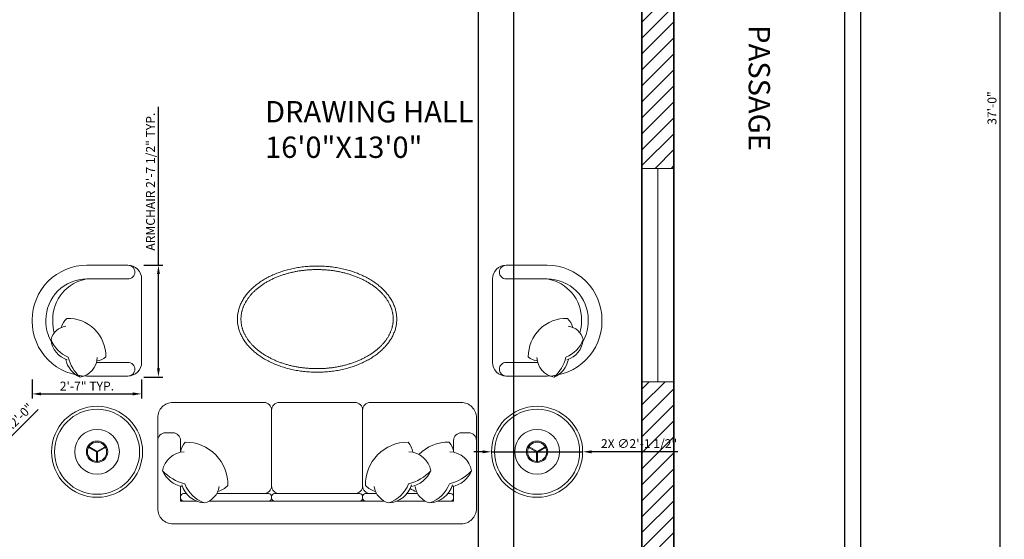
# Model space of a CAD drawing. Units: inches. Extents: x 3618 to 4156, y 1271 to 2023.
# Tile 3 of 5: x 3879 to 4156, y 1488 to 1635. Entities that reach past the tile are written whole.
import ezdxf

# ---------------------------------------------------------------- set-up
doc = ezdxf.new("R2010")
doc.units = ezdxf.units.IN
for name, color, linetype, lineweight in [('A-ANNO-DIMS', 2, 'Continuous', 18), ('A-AREA-IDEN', 7, 'Continuous', 18), ('A-FURN', 8, 'Continuous', 18), ('A-GLAZ', 4, 'Continuous', 18), ('A-WALL', 7, 'Continuous', 35), ('A-WALL-PATT', 252, 'Continuous', 13), ('C-PROP', 7, 'Continuous', 25)]:
    doc.layers.add(name, color=color, linetype=linetype, lineweight=lineweight)
doc.styles.get("Standard").update_dxf_attribs({"font": 'arial.ttf'})
doc.dimstyles.new('ISO-25', dxfattribs={"dimtxt": 2.5, "dimasz": 2.5, "dimexe": 1.25, "dimexo": 0.625, "dimtad": 1, "dimdec": 0, "dimlunit": 3, "dimtxsty": 'Standard', "dimcen": 2.5, "dimadec": 0, "dimazin": 0, "dimtfac": 1, "dimtdec": 0, "dimtmove": 0, "dimatfit": 3, "dimfxl": 1, "dimarcsym": 0})

# ---------------------------------------------------------------- blocks, each defined once
blk = doc.blocks.new('WINDOW-60X9')
for p, q in [((0, 60), (0, 0)), ((9, 60), (0, 60)), ((4.5, 60), (4.5, 0)), ((9, 0), (9, 60)), ((0, 0), (9, 0))]:
    blk.add_line(p, q)
blk = doc.blocks.new('ARMCHAIR')
at = {"ltscale": 0.03}
blk.add_lwpolyline([(30.78, 15.9), (30.78, 27.63, 0.414214), (26.93, 31.48), (15.39, 31.48, 0.414214), (0, 16.09), (0, 15.9), (0, 15.71, 0.414214), (15.39, 0.31), (26.93, 0.31, 0.414214), (30.78, 4.16), (30.78, 15.9)], format="xyb", dxfattribs=at)
for points in [[(15.39, 27.63), (26.93, 27.63, 0.414214), (28.86, 29.56), (28.86, 29.56, 0.414214), (26.93, 31.48)], [(15.39, 27.63, 0.414214), (3.85, 16.09), (3.85, 15.9)], [(15.39, 27.63, 0.372719), (5.77, 16.09), (5.77, 15.9)], [(5.37, 9.98, -0.130591), (3.85, 15.71), (3.85, 15.9)], [(9.88, 4.85, -0.306663), (5.29, 10.58, -0.30633), (9.48, 14.33, 0.872847)], [(6.19, 12.43, -0.072384), (5.77, 15.71), (5.77, 15.9)], [(18.18, 4.54, 0.165541), (20.72, 5.73, 0.425989), (9.7, 16.54, 0.121523), (8.18, 13.97, -7.115464)], [(13.45, 0, -0.14773), (10.14, 5.62, -0.213343), (5.29, 10.58, -0.178662)], [(18.3, 5.51, -0.356772), (13.45, 0, -0.249542), (9.45, 4.99, 9.61688)], [(18.09, 4.16), (26.93, 4.16, -0.414214), (28.86, 2.24), (28.86, 2.24, -0.414214), (26.93, 0.31)]]:
    blk.add_lwpolyline(points, format="xyb")
blk = doc.blocks.new('TABLE-END-ROUND')
at = {"ltscale": 0.03}
for p, q in [((-0.07, -0.12), (-2.67, 1.39)), ((0.07, 0.12), (-2.54, 1.62)), ((-0.13, 0), (-0.13, -3.01)), ((-0.07, 0.12), (2.54, 1.62)), ((0.07, -0.12), (2.67, 1.39)), ((0.13, 0), (0.13, -3.01))]:
    blk.add_line(p, q, dxfattribs=at)
for radius in [12.8, 6.29, 3.01, 2.7]:
    blk.add_circle((0, 0), radius, dxfattribs=at)
blk.add_circle((0, 0), 11.95)
blk = doc.blocks.new('*D40')
at = {"layer": 'A-ANNO-DIMS', "color": 0, "lineweight": -2, "transparency": 16777216}
for p, q in [((3918.22, 1565.57), (3918.22, 1610.13)), ((3914.12, 1565.57), (3919.47, 1565.57)), ((3918.22, 1536.59), (3918.22, 1563.07)), ((3914.12, 1534.09), (3919.47, 1534.09))]:
    blk.add_line(p, q, dxfattribs=at)
at = {"layer": 'A-ANNO-DIMS', "color": 0, "transparency": 16777216}
for points in [[(3917.81, 1563.07), (3918.64, 1563.07), (3918.22, 1565.57)], [(3917.81, 1536.59), (3918.64, 1536.59), (3918.22, 1534.09)]]:
    blk.add_solid(points, dxfattribs=at)
at = {"layer": 'Defpoints', "color": 0, "transparency": 16777216}
for p in [(3913.5, 1565.57), (3918.22, 1565.57), (3913.5, 1534.09)]:
    blk.add_point(p, dxfattribs=at)
at = {"layer": 'A-ANNO-DIMS', "color": 0, "transparency": 16777216, "insert": (3916.3, 1589.1), "char_height": 2.5, "attachment_point": 5, "rotation": 90}
blk.add_mtext('ARMCHAIR 2\'-7 1/2" TYP.', dxfattribs=at)
blk = doc.blocks.new('*D41')
at = {"layer": 'A-ANNO-DIMS', "color": 0, "lineweight": -2, "transparency": 16777216}
for p, q in [((3882.72, 1533.47), (3882.72, 1528.12)), ((3913.5, 1533.47), (3913.5, 1528.12)), ((3885.22, 1529.37), (3911, 1529.37))]:
    blk.add_line(p, q, dxfattribs=at)
at = {"layer": 'A-ANNO-DIMS', "color": 0, "transparency": 16777216}
for points in [[(3885.22, 1529.79), (3885.22, 1528.95), (3882.72, 1529.37)], [(3911, 1529.79), (3911, 1528.95), (3913.5, 1529.37)]]:
    blk.add_solid(points, dxfattribs=at)
at = {"layer": 'Defpoints', "color": 0, "transparency": 16777216}
for p in [(3882.72, 1534.09), (3913.5, 1534.09), (3913.5, 1529.37)]:
    blk.add_point(p, dxfattribs=at)
at = {"layer": 'A-ANNO-DIMS', "color": 0, "transparency": 16777216, "insert": (3898.11, 1531.25), "char_height": 2.5, "attachment_point": 5}
blk.add_mtext('2\'-7" TYP.', dxfattribs=at)
blk = doc.blocks.new('*D53')
at = {"layer": 'A-ANNO-DIMS', "color": 0, "lineweight": -2, "transparency": 16777216}
for p, q in [((4008.19, 1440.44), (4008.19, 1974.21)), ((4018.19, 1440.44), (4018.19, 1974.21)), ((4010.69, 1972.96), (4015.69, 1972.96))]:
    blk.add_line(p, q, dxfattribs=at)
at = {"layer": 'A-ANNO-DIMS', "color": 0, "transparency": 16777216}
for points in [[(4010.69, 1973.38), (4010.69, 1972.54), (4008.19, 1972.96)], [(4015.69, 1973.38), (4015.69, 1972.54), (4018.19, 1972.96)]]:
    blk.add_solid(points, dxfattribs=at)
at = {"layer": 'Defpoints', "color": 0, "transparency": 16777216}
for p in [(4018.19, 1972.96), (4008.19, 1439.81), (4018.19, 1439.81)]:
    blk.add_point(p, dxfattribs=at)
at = {"layer": 'A-ANNO-DIMS', "color": 0, "transparency": 16777216, "insert": (4013.19, 1974.86), "char_height": 2.5, "attachment_point": 5}
blk.add_mtext('0\'-10"', dxfattribs=at)
blk = doc.blocks.new('*D56')
at = {"layer": 'A-ANNO-DIMS', "color": 0, "lineweight": -2, "transparency": 16777216}
for p, q in [((4063.81, 1831.81), (4156.09, 1831.81)), ((4154.84, 1829.31), (4154.84, 1390.31)), ((4063.81, 1387.81), (4156.09, 1387.81))]:
    blk.add_line(p, q, dxfattribs=at)
at = {"layer": 'A-ANNO-DIMS', "color": 0, "transparency": 16777216}
for points in [[(4154.42, 1829.31), (4155.25, 1829.31), (4154.84, 1831.81)], [(4154.42, 1390.31), (4155.25, 1390.31), (4154.84, 1387.81)]]:
    blk.add_solid(points, dxfattribs=at)
at = {"layer": 'Defpoints', "color": 0, "transparency": 16777216}
for p in [(4063.19, 1831.81), (4063.19, 1387.81), (4154.84, 1387.81)]:
    blk.add_point(p, dxfattribs=at)
at = {"layer": 'A-ANNO-DIMS', "color": 0, "transparency": 16777216, "insert": (4152.94, 1609.81), "char_height": 2.5, "attachment_point": 5, "rotation": 90}
blk.add_mtext('37\'-0"', dxfattribs=at)
blk = doc.blocks.new('*D60')
at = {"layer": 'A-ANNO-DIMS', "color": 0, "lineweight": -2, "transparency": 16777216}
for p, q in [((4009.41, 1513.08), (4006.91, 1513.08)), ((4011.91, 1513.08), (4037.51, 1513.08)), ((4064.24, 1513.08), (4040.01, 1513.08))]:
    blk.add_line(p, q, dxfattribs=at)
at = {"layer": 'A-ANNO-DIMS', "color": 0, "transparency": 16777216}
for points in [[(4009.41, 1513.49), (4009.41, 1512.66), (4011.91, 1513.08)], [(4040.01, 1513.49), (4040.01, 1512.66), (4037.51, 1513.08)]]:
    blk.add_solid(points, dxfattribs=at)
at = {"layer": 'Defpoints', "color": 0, "transparency": 16777216}
for p in [(4011.91, 1513.08), (4037.51, 1513.08)]:
    blk.add_point(p, dxfattribs=at)
at = {"layer": 'A-ANNO-DIMS', "color": 0, "transparency": 16777216, "insert": (4053.38, 1515.05), "char_height": 2.5, "attachment_point": 5, "rotation": 359.9984}
blk.add_mtext('2X ∅2\'-1 1/2"', dxfattribs=at)
blk = doc.blocks.new('*D62')
at = {"layer": 'A-ANNO-DIMS', "color": 0, "lineweight": -2, "transparency": 16777216}
for p, q in [((3884.38, 1525), (3870.43, 1511.05)), ((3851.69, 1492.31), (3868.66, 1509.28))]:
    blk.add_line(p, q, dxfattribs=at)
at = {"layer": 'A-ANNO-DIMS', "color": 0, "transparency": 16777216}
blk.add_solid([(3870.13, 1511.34), (3870.72, 1510.75), (3868.66, 1509.28)], dxfattribs=at)
at = {"layer": 'Defpoints', "color": 0, "transparency": 16777216}
for p in [(3868.66, 1509.28), (3851.69, 1492.31)]:
    blk.add_point(p, dxfattribs=at)
at = {"layer": 'A-ANNO-DIMS', "color": 0, "transparency": 16777216, "insert": (3877.5, 1520.81), "char_height": 2.5, "attachment_point": 5, "rotation": 45.0011}
blk.add_mtext('3X R2\'-0"', dxfattribs=at)

msp = doc.modelspace()

# ---------------------------------------------------------------- hatches: boundary and pattern name
at = {"layer": 'A-WALL-PATT'}
h = msp.add_hatch(dxfattribs=at)
h.set_pattern_fill('ANSI31', color=256)
h.paths.add_polyline_path([(4115.69, 1933.81), (3704.69, 1933.81), (3704.69, 1885.81), (3713.69, 1885.81), (3713.69, 1924.81), (4115.69, 1924.81)])
h.paths.add_polyline_path([(3886.19, 1924.81), (3881.69, 1924.81), (3881.69, 1786.81), (3875.69, 1786.81), (3875.69, 1782.31), (3892.19, 1782.31), (3892.19, 1786.81), (3886.19, 1786.81)])
h.paths.add_polyline_path([(3763.69, 1784.56), (3763.69, 1786.81), (3713.69, 1786.81), (3713.69, 1782.31), (3763.69, 1782.31)], flags=17)
h.paths.add_polyline_path([(3713.69, 1825.81), (3704.69, 1825.81), (3704.69, 1764.31), (3713.69, 1764.31)])
h.paths.add_polyline_path([(3802.19, 1782.31), (3835.69, 1782.31), (3835.69, 1784.56), (3835.69, 1786.81), (3791.69, 1786.81), (3791.69, 1782.31), (3797.69, 1782.31), (3797.69, 1722.31), (3713.69, 1722.31), (3713.69, 1717.81), (3797.69, 1717.81), (3797.69, 1657.81), (3791.69, 1657.81), (3791.69, 1653.31), (3851.69, 1653.31), (3851.69, 1647.31), (3856.19, 1647.31), (3856.19, 1657.81), (3802.19, 1657.81)])
h.paths.add_polyline_path([(3713.69, 1740.31), (3704.69, 1740.31), (3704.69, 1699.81), (3713.69, 1699.81)])
h.paths.add_polyline_path([(3713.69, 1675.81), (3704.69, 1675.81), (3704.69, 1623.31), (3713.69, 1623.31)])
h.paths.add_polyline_path([(3743.18, 1533.31), (3713.69, 1533.31), (3713.69, 1563.31), (3704.69, 1563.31), (3704.69, 1524.31), (3743.18, 1524.31)])
h.paths.add_polyline_path([(3856.19, 1533.31), (3803.18, 1533.31), (3803.18, 1524.31), (3847.19, 1524.31), (3847.19, 1518.31), (3856.19, 1518.31)])
h.paths.add_polyline_path([(3856.19, 1607.31), (3853.94, 1607.31), (3851.69, 1607.31), (3851.69, 1533.31), (3856.19, 1533.31)])
h.paths.add_polyline_path([(3763.69, 1655.56), (3763.69, 1657.81), (3713.69, 1657.81), (3713.69, 1653.31), (3763.69, 1653.31)], flags=17)
h.paths.add_polyline_path([(4063.19, 1670.56), (4054.19, 1670.56), (4054.19, 1645.31), (3940.98, 1645.31), (3940.98, 1640.81), (4054.19, 1640.81), (4054.19, 1592.81), (4063.19, 1592.81)])
h.paths.add_polyline_path([(4063.19, 1532.81), (4054.19, 1532.81), (4054.19, 1454.31), (4063.19, 1454.31)])
h.paths.add_polyline_path([(4054.19, 1484.81), (3985.19, 1484.81), (3985.19, 1475.81), (4054.19, 1475.81)])
h.paths.add_polyline_path([(3925.19, 1484.81), (3856.19, 1484.81), (3856.19, 1490.81), (3847.19, 1490.81), (3847.19, 1475.81), (3925.19, 1475.81)])
h.paths.add_polyline_path([(4063.19, 1396.81), (3928.19, 1396.81), (3928.19, 1387.81), (4063.19, 1387.81)])
h.paths.add_polyline_path([(4063.19, 1418.31), (4054.19, 1418.31), (4054.19, 1396.81), (4063.19, 1396.81)])
h.paths.add_polyline_path([(4063.19, 1790.42), (4054.19, 1790.42), (4054.19, 1786.81), (3932.19, 1786.81), (3932.19, 1784.56), (3932.19, 1782.31), (4054.19, 1782.31), (4054.19, 1771.81), (4063.19, 1771.81)])
h.paths.add_polyline_path([(4070.69, 1840.81), (4058.69, 1840.81), (4058.69, 1890.81), (4056.44, 1890.81), (4054.19, 1890.81), (4054.19, 1826.42), (4063.19, 1826.42), (4063.19, 1831.81), (4070.69, 1831.81)])
h.paths.add_polyline_path([(4115.69, 1924.81), (4106.69, 1924.81), (4106.69, 1840.81), (4094.69, 1840.81), (4094.69, 1831.81), (4115.69, 1831.81)])
h.paths.add_polyline_path([(4063.19, 1731.81), (4058.69, 1731.81), (4054.19, 1731.81), (4054.19, 1706.56), (4063.19, 1706.56)])

# ---------------------------------------------------------------- linework, layer by layer
at = {"layer": 'A-FURN', "ltscale": 0.03}
msp.add_lwpolyline([(3918.03, 1522.68, -0.414214), (3922.29, 1526.95), (3947.9, 1526.95, -0.414214), (3950.03, 1524.81, -0.414214), (3952.17, 1526.95), (3973.5, 1526.95, -0.414214), (3975.64, 1524.81, -0.414214), (3977.77, 1526.95), (4003.37, 1526.95, -0.414214), (4007.64, 1522.68), (4007.64, 1497.07, -0.414214), (4003.37, 1492.81), (3922.29, 1492.81, -0.414214), (3918.03, 1497.07)], format="xyb", close=True, dxfattribs=at)
at = {"layer": 'A-FURN'}
for points in [[(3947.9, 1501.34, 0.414214), (3950.03, 1503.48), (3950.03, 1524.81, 0.414214)], [(3977.77, 1501.34, -0.414214), (3975.64, 1503.48), (3975.64, 1524.81, -0.414214)], [(3918.03, 1516.28, -0.414214), (3920.16, 1518.41), (3922.29, 1518.41, -0.414214), (3924.43, 1516.28), (3924.43, 1512.97)], [(4001.24, 1512.97), (4001.24, 1516.28, -0.414214), (4003.37, 1518.41), (4005.51, 1518.41, -0.414214), (4007.64, 1516.28)], [(3924.42, 1512.97, -0.165541), (3925.74, 1515.79, -0.425989), (3937.73, 1503.57, -0.121523), (3934.88, 1501.88, 7.115464)], [(3989.75, 1512.97, 0.165541), (3988.43, 1515.79, 0.425989), (3976.45, 1503.57, 0.121523), (3979.29, 1501.88, -7.115464)], [(4001.25, 1512.97, 0.165541), (3999.93, 1515.79, 0.200231), (3991.46, 1512.36, 0.121523)], [(3925.5, 1513.1, 0.356772), (3919.38, 1507.72, 0.249542), (3924.92, 1503.29, -9.61688)], [(3988.68, 1513.1, -0.356772), (3994.79, 1507.72, -0.249542), (3989.25, 1503.29, 9.61688)], [(4000.17, 1513.1, -0.356772), (4006.28, 1507.72, -0.249542), (4000.74, 1503.29, 9.61688)], [(3919.38, 1507.72, 0.14773), (3925.62, 1504.06, 0.213343), (3931.12, 1498.68, 0.178662)], [(3994.79, 1507.72, -0.14773), (3988.55, 1504.06, -0.213343), (3983.05, 1498.68, -0.178662)], [(4006.28, 1507.72, -0.14773), (4000.05, 1504.06, -0.213343), (3994.55, 1498.68, -0.178662)], [(3924.76, 1503.76, 0.306663), (3931.12, 1498.68, 0.30633), (3935.28, 1503.32, -0.872847)], [(3989.42, 1503.76, -0.306663), (3983.05, 1498.68, -0.30633), (3978.89, 1503.32, 0.872847)], [(4000.91, 1503.76, -0.306663), (3994.55, 1498.68, -0.30633), (3990.39, 1503.32, 0.872847)], [(3926.06, 1501.34), (3925.28, 1501.34, 0.414214), (3924.43, 1500.49), (3924.43, 1500.06, 0.414214), (3925.28, 1499.21)], [(3932.47, 1499.21), (3949.18, 1499.21, 0.414214), (3950.03, 1500.06), (3950.03, 1500.49, 0.414214), (3949.18, 1501.34), (3934.61, 1501.34, 0.414214)], [(3952.17, 1501.34, -0.414214), (3950.03, 1503.48)], [(3973.5, 1501.34, 0.414214), (3975.64, 1503.48)], [(3981.71, 1499.21), (3976.49, 1499.21, -0.414214), (3975.64, 1500.06), (3975.64, 1500.49, -0.414214), (3976.49, 1501.34), (3979.56, 1501.34, -0.414214)], [(3988.12, 1501.34), (3991.05, 1501.34, -0.414214)], [(3989, 1502.72, 0.071865), (3990.79, 1501.88, -7.115464)], [(3996.75, 1499.21), (4001.24, 1499.21), (4001.24, 1503.4, -0.414214)], [(3999.61, 1501.34), (4000.39, 1501.34, -0.414214), (4001.24, 1500.49), (4001.24, 1500.06, -0.414214), (4000.39, 1499.21)], [(3925.28, 1499.21), (3928.92, 1499.21, 0.414214)], [(3993.2, 1499.21), (3985.26, 1499.21, -0.414214)], [(4000.39, 1499.21), (3996.75, 1499.21, -0.414214)]]:
    msp.add_lwpolyline(points, format="xyb", dxfattribs=at)
for points in [[(3924.43, 1503.4), (3924.43, 1499.21), (3928.92, 1499.21)], [(3932.47, 1499.21), (3981.71, 1499.21)], [(3985.26, 1499.21), (3993.2, 1499.21)]]:
    msp.add_lwpolyline(points, dxfattribs=at)
msp.add_lwpolyline([(3974.78, 1499.21), (3950.89, 1499.21, -0.414214), (3950.03, 1500.06), (3950.03, 1500.49, -0.414214), (3950.89, 1501.34), (3974.78, 1501.34, -0.414214), (3975.64, 1500.49), (3975.64, 1500.06, -0.414214)], format="xyb", close=True, dxfattribs=at)
at = {"layer": 'A-FURN', "ltscale": 0.03}
msp.add_polyline3d([(3940.43, 1550.42, 0), (3940.43, 1550.13, 0), (3940.45, 1549.85, 0), (3940.47, 1549.57, 0), (3940.49, 1549.29, 0), (3940.53, 1549.01, 0), (3940.57, 1548.73, 0), (3940.63, 1548.44, 0), (3940.69, 1548.16, 0), (3940.75, 1547.89, 0), (3940.83, 1547.61, 0), (3940.91, 1547.33, 0), (3941.01, 1547.05, 0), (3941.1, 1546.78, 0), (3941.21, 1546.51, 0), (3941.33, 1546.23, 0), (3941.45, 1545.96, 0), (3941.58, 1545.69, 0), (3941.72, 1545.43, 0), (3941.86, 1545.16, 0), (3942.02, 1544.9, 0), (3942.18, 1544.64, 0), (3942.34, 1544.38, 0), (3942.52, 1544.12, 0), (3942.7, 1543.86, 0), (3942.89, 1543.61, 0), (3943.09, 1543.36, 0), (3943.29, 1543.11, 0), (3943.5, 1542.87, 0), (3943.72, 1542.63, 0), (3943.94, 1542.39, 0), (3944.18, 1542.15, 0), (3944.41, 1541.92, 0), (3944.66, 1541.68, 0), (3944.91, 1541.46, 0), (3945.17, 1541.23, 0), (3945.43, 1541.01, 0), (3945.7, 1540.79, 0), (3945.98, 1540.58, 0), (3946.26, 1540.37, 0), (3946.55, 1540.16, 0), (3946.84, 1539.96, 0), (3947.14, 1539.76, 0), (3947.45, 1539.56, 0), (3947.76, 1539.37, 0), (3948.08, 1539.18, 0), (3948.4, 1539, 0), (3948.72, 1538.82, 0), (3949.06, 1538.64, 0), (3949.39, 1538.47, 0), (3949.73, 1538.3, 0), (3950.08, 1538.14, 0), (3950.43, 1537.98, 0), (3950.79, 1537.82, 0), (3951.15, 1537.68, 0), (3951.51, 1537.53, 0), (3951.88, 1537.39, 0), (3952.25, 1537.25, 0), (3952.62, 1537.12, 0), (3953, 1537, 0), (3953.39, 1536.87, 0), (3953.77, 1536.76, 0), (3954.16, 1536.65, 0), (3954.55, 1536.54, 0), (3954.95, 1536.44, 0), (3955.35, 1536.34, 0), (3955.75, 1536.25, 0), (3956.15, 1536.16, 0), (3956.56, 1536.08, 0), (3956.97, 1536, 0), (3957.38, 1535.93, 0), (3957.79, 1535.86, 0), (3958.2, 1535.8, 0), (3958.62, 1535.75, 0), (3959.04, 1535.7, 0), (3959.45, 1535.65, 0), (3959.87, 1535.61, 0), (3960.3, 1535.58, 0), (3960.72, 1535.55, 0), (3961.14, 1535.52, 0), (3961.56, 1535.51, 0), (3961.99, 1535.49, 0), (3962.41, 1535.48, 0), (3962.83, 1535.48, 0), (3963.26, 1535.48, 0), (3963.68, 1535.49, 0), (3964.11, 1535.51, 0), (3964.53, 1535.52, 0), (3964.95, 1535.55, 0), (3965.37, 1535.58, 0), (3965.79, 1535.61, 0), (3966.21, 1535.65, 0), (3966.63, 1535.7, 0), (3967.05, 1535.75, 0), (3967.46, 1535.8, 0), (3967.88, 1535.86, 0), (3968.29, 1535.93, 0), (3968.7, 1536, 0), (3969.11, 1536.08, 0), (3969.51, 1536.16, 0), (3969.92, 1536.25, 0), (3970.32, 1536.34, 0), (3970.72, 1536.44, 0), (3971.11, 1536.54, 0), (3971.51, 1536.65, 0), (3971.89, 1536.76, 0), (3972.28, 1536.87, 0), (3972.66, 1537, 0), (3973.04, 1537.12, 0), (3973.42, 1537.25, 0), (3973.79, 1537.39, 0), (3974.16, 1537.53, 0), (3974.52, 1537.68, 0), (3974.88, 1537.82, 0), (3975.24, 1537.98, 0), (3975.59, 1538.14, 0), (3975.93, 1538.3, 0), (3976.28, 1538.47, 0), (3976.61, 1538.64, 0), (3976.94, 1538.82, 0), (3977.27, 1539, 0), (3977.59, 1539.18, 0), (3977.91, 1539.37, 0), (3978.22, 1539.56, 0), (3978.53, 1539.76, 0), (3978.83, 1539.96, 0), (3979.12, 1540.16, 0), (3979.41, 1540.37, 0), (3979.69, 1540.58, 0), (3979.97, 1540.79, 0), (3980.24, 1541.01, 0), (3980.5, 1541.23, 0), (3980.76, 1541.46, 0), (3981.01, 1541.68, 0), (3981.25, 1541.92, 0), (3981.49, 1542.15, 0), (3981.72, 1542.39, 0), (3981.95, 1542.63, 0), (3982.17, 1542.87, 0), (3982.38, 1543.11, 0), (3982.58, 1543.36, 0), (3982.78, 1543.61, 0), (3982.97, 1543.86, 0), (3983.15, 1544.12, 0), (3983.32, 1544.38, 0), (3983.49, 1544.64, 0), (3983.65, 1544.9, 0), (3983.81, 1545.16, 0), (3983.95, 1545.43, 0), (3984.09, 1545.69, 0), (3984.22, 1545.96, 0), (3984.34, 1546.23, 0), (3984.46, 1546.51, 0), (3984.56, 1546.78, 0), (3984.66, 1547.05, 0), (3984.75, 1547.33, 0), (3984.84, 1547.61, 0), (3984.91, 1547.89, 0), (3984.98, 1548.16, 0), (3985.04, 1548.44, 0), (3985.09, 1548.73, 0), (3985.14, 1549.01, 0), (3985.17, 1549.29, 0), (3985.2, 1549.57, 0), (3985.22, 1549.85, 0), (3985.23, 1550.13, 0), (3985.24, 1550.42, 0), (3985.23, 1550.7, 0), (3985.22, 1550.98, 0), (3985.2, 1551.27, 0), (3985.17, 1551.55, 0), (3985.14, 1551.83, 0), (3985.09, 1552.11, 0), (3985.04, 1552.39, 0), (3984.98, 1552.67, 0), (3984.91, 1552.95, 0), (3984.84, 1553.23, 0), (3984.75, 1553.5, 0), (3984.66, 1553.78, 0), (3984.56, 1554.06, 0), (3984.46, 1554.33, 0), (3984.34, 1554.6, 0), (3984.22, 1554.87, 0), (3984.09, 1555.14, 0), (3983.95, 1555.41, 0), (3983.81, 1555.67, 0), (3983.65, 1555.94, 0), (3983.49, 1556.2, 0), (3983.32, 1556.46, 0), (3983.15, 1556.72, 0), (3982.97, 1556.97, 0), (3982.78, 1557.22, 0), (3982.58, 1557.47, 0), (3982.38, 1557.72, 0), (3982.17, 1557.97, 0), (3981.95, 1558.21, 0), (3981.72, 1558.45, 0), (3981.49, 1558.69, 0), (3981.25, 1558.92, 0), (3981.01, 1559.15, 0), (3980.76, 1559.38, 0), (3980.5, 1559.6, 0), (3980.24, 1559.82, 0), (3979.97, 1560.04, 0), (3979.69, 1560.26, 0), (3979.41, 1560.47, 0), (3979.12, 1560.67, 0), (3978.83, 1560.88, 0), (3978.53, 1561.08, 0), (3978.22, 1561.27, 0), (3977.91, 1561.47, 0), (3977.59, 1561.65, 0), (3977.27, 1561.84, 0), (3976.94, 1562.02, 0), (3976.61, 1562.2, 0), (3976.28, 1562.37, 0), (3975.93, 1562.53, 0), (3975.59, 1562.7, 0), (3975.24, 1562.86, 0), (3974.88, 1563.01, 0), (3974.52, 1563.16, 0), (3974.16, 1563.31, 0), (3973.79, 1563.45, 0), (3973.42, 1563.58, 0), (3973.04, 1563.71, 0), (3972.66, 1563.84, 0), (3972.28, 1563.96, 0), (3971.89, 1564.08, 0), (3971.51, 1564.19, 0), (3971.11, 1564.3, 0), (3970.72, 1564.4, 0), (3970.32, 1564.5, 0), (3969.92, 1564.59, 0), (3969.51, 1564.67, 0), (3969.11, 1564.76, 0), (3968.7, 1564.83, 0), (3968.29, 1564.9, 0), (3967.88, 1564.97, 0), (3967.46, 1565.03, 0), (3967.05, 1565.09, 0), (3966.63, 1565.14, 0), (3966.21, 1565.18, 0), (3965.79, 1565.22, 0), (3965.37, 1565.26, 0), (3964.95, 1565.29, 0), (3964.53, 1565.31, 0), (3964.11, 1565.33, 0), (3963.68, 1565.34, 0), (3963.26, 1565.35, 0), (3962.83, 1565.35, 0), (3962.41, 1565.35, 0), (3961.99, 1565.34, 0), (3961.56, 1565.33, 0), (3961.14, 1565.31, 0), (3960.72, 1565.29, 0), (3960.3, 1565.26, 0), (3959.87, 1565.22, 0), (3959.45, 1565.18, 0), (3959.04, 1565.14, 0), (3958.62, 1565.09, 0), (3958.2, 1565.03, 0), (3957.79, 1564.97, 0), (3957.38, 1564.9, 0), (3956.97, 1564.83, 0), (3956.56, 1564.76, 0), (3956.15, 1564.67, 0), (3955.75, 1564.59, 0), (3955.35, 1564.5, 0), (3954.95, 1564.4, 0), (3954.55, 1564.3, 0), (3954.16, 1564.19, 0), (3953.77, 1564.08, 0), (3953.39, 1563.96, 0), (3953, 1563.84, 0), (3952.62, 1563.71, 0), (3952.25, 1563.58, 0), (3951.88, 1563.45, 0), (3951.51, 1563.31, 0), (3951.15, 1563.16, 0), (3950.79, 1563.01, 0), (3950.43, 1562.86, 0), (3950.08, 1562.7, 0), (3949.73, 1562.53, 0), (3949.39, 1562.37, 0), (3949.06, 1562.2, 0), (3948.72, 1562.02, 0), (3948.4, 1561.84, 0), (3948.08, 1561.65, 0), (3947.76, 1561.47, 0), (3947.45, 1561.27, 0), (3947.14, 1561.08, 0), (3946.84, 1560.88, 0), (3946.55, 1560.67, 0), (3946.26, 1560.47, 0), (3945.98, 1560.26, 0), (3945.7, 1560.04, 0), (3945.43, 1559.82, 0), (3945.17, 1559.6, 0), (3944.91, 1559.38, 0), (3944.66, 1559.15, 0), (3944.41, 1558.92, 0), (3944.18, 1558.69, 0), (3943.94, 1558.45, 0), (3943.72, 1558.21, 0), (3943.5, 1557.97, 0), (3943.29, 1557.72, 0), (3943.09, 1557.47, 0), (3942.89, 1557.22, 0), (3942.7, 1556.97, 0), (3942.52, 1556.72, 0), (3942.34, 1556.46, 0), (3942.18, 1556.2, 0), (3942.02, 1555.94, 0), (3941.86, 1555.67, 0), (3941.72, 1555.41, 0), (3941.58, 1555.14, 0), (3941.45, 1554.87, 0), (3941.33, 1554.6, 0), (3941.21, 1554.33, 0), (3941.1, 1554.06, 0), (3941.01, 1553.78, 0), (3940.91, 1553.5, 0), (3940.83, 1553.23, 0), (3940.75, 1552.95, 0), (3940.69, 1552.67, 0), (3940.63, 1552.39, 0), (3940.57, 1552.11, 0), (3940.53, 1551.83, 0), (3940.49, 1551.55, 0), (3940.47, 1551.27, 0), (3940.45, 1550.98, 0), (3940.43, 1550.7, 0), (3940.43, 1550.42, 0)], dxfattribs=at)
at = {"layer": 'A-FURN'}
msp.add_polyline3d([(3941.43, 1550.42, 0), (3941.43, 1550.26, 0), (3941.43, 1550.11, 0), (3941.44, 1549.96, 0), (3941.45, 1549.8, 0), (3941.46, 1549.65, 0), (3941.47, 1549.49, 0), (3941.49, 1549.33, 0), (3941.51, 1549.18, 0), (3941.54, 1549.02, 0), (3941.56, 1548.86, 0), (3941.59, 1548.7, 0), (3941.62, 1548.54, 0), (3941.66, 1548.38, 0), (3941.7, 1548.22, 0), (3941.74, 1548.06, 0), (3941.78, 1547.9, 0), (3941.83, 1547.74, 0), (3941.88, 1547.58, 0), (3941.93, 1547.42, 0), (3941.99, 1547.25, 0), (3942.05, 1547.09, 0), (3942.12, 1546.93, 0), (3942.18, 1546.76, 0), (3942.25, 1546.6, 0), (3942.33, 1546.44, 0), (3942.4, 1546.27, 0), (3942.49, 1546.11, 0), (3942.57, 1545.95, 0), (3942.66, 1545.78, 0), (3942.75, 1545.62, 0), (3942.84, 1545.46, 0), (3942.94, 1545.29, 0), (3943.04, 1545.13, 0), (3943.15, 1544.97, 0), (3943.26, 1544.81, 0), (3943.37, 1544.65, 0), (3943.48, 1544.48, 0), (3943.6, 1544.32, 0), (3943.72, 1544.16, 0), (3943.85, 1544, 0), (3943.98, 1543.85, 0), (3944.11, 1543.69, 0), (3944.25, 1543.53, 0), (3944.39, 1543.38, 0), (3944.53, 1543.22, 0), (3944.68, 1543.07, 0), (3944.83, 1542.91, 0), (3944.98, 1542.76, 0), (3945.14, 1542.61, 0), (3945.3, 1542.46, 0), (3945.46, 1542.31, 0), (3945.63, 1542.16, 0), (3945.8, 1542.01, 0), (3945.98, 1541.87, 0), (3946.15, 1541.72, 0), (3946.33, 1541.58, 0), (3946.52, 1541.43, 0), (3946.7, 1541.29, 0), (3946.89, 1541.15, 0), (3947.09, 1541.02, 0), (3947.28, 1540.88, 0), (3947.48, 1540.74, 0), (3947.68, 1540.61, 0), (3947.88, 1540.48, 0), (3948.09, 1540.35, 0), (3948.3, 1540.22, 0), (3948.51, 1540.09, 0), (3948.72, 1539.97, 0), (3948.94, 1539.85, 0), (3949.16, 1539.73, 0), (3949.38, 1539.61, 0), (3949.6, 1539.49, 0), (3949.82, 1539.37, 0), (3950.05, 1539.26, 0), (3950.28, 1539.15, 0), (3950.51, 1539.04, 0), (3950.75, 1538.93, 0), (3950.98, 1538.83, 0), (3951.22, 1538.72, 0), (3951.46, 1538.62, 0), (3951.7, 1538.53, 0), (3951.94, 1538.43, 0), (3952.19, 1538.34, 0), (3952.43, 1538.25, 0), (3952.68, 1538.16, 0), (3952.92, 1538.07, 0), (3953.17, 1537.99, 0), (3953.42, 1537.91, 0), (3953.67, 1537.83, 0), (3953.92, 1537.75, 0), (3954.17, 1537.68, 0), (3954.42, 1537.61, 0), (3954.67, 1537.54, 0), (3954.92, 1537.47, 0), (3955.17, 1537.4, 0), (3955.43, 1537.34, 0), (3955.68, 1537.28, 0), (3955.93, 1537.22, 0), (3956.19, 1537.17, 0), (3956.44, 1537.11, 0), (3956.7, 1537.06, 0), (3956.95, 1537.01, 0), (3957.21, 1536.97, 0), (3957.46, 1536.92, 0), (3957.72, 1536.88, 0), (3957.98, 1536.84, 0), (3958.24, 1536.8, 0), (3958.49, 1536.76, 0), (3958.75, 1536.73, 0), (3959.01, 1536.7, 0), (3959.27, 1536.67, 0), (3959.53, 1536.64, 0), (3959.78, 1536.62, 0), (3960.04, 1536.59, 0), (3960.3, 1536.57, 0), (3960.56, 1536.55, 0), (3960.82, 1536.54, 0), (3961.08, 1536.52, 0), (3961.34, 1536.51, 0), (3961.6, 1536.5, 0), (3961.86, 1536.49, 0), (3962.12, 1536.48, 0), (3962.38, 1536.48, 0), (3962.64, 1536.48, 0), (3962.9, 1536.48, 0), (3963.16, 1536.48, 0), (3963.42, 1536.48, 0), (3963.68, 1536.49, 0), (3963.94, 1536.5, 0), (3964.2, 1536.5, 0), (3964.46, 1536.52, 0), (3964.72, 1536.53, 0), (3964.98, 1536.55, 0), (3965.24, 1536.56, 0), (3965.5, 1536.58, 0), (3965.75, 1536.61, 0), (3966.01, 1536.63, 0), (3966.27, 1536.66, 0), (3966.53, 1536.68, 0), (3966.79, 1536.71, 0), (3967.05, 1536.75, 0), (3967.3, 1536.78, 0), (3967.56, 1536.82, 0), (3967.82, 1536.86, 0), (3968.08, 1536.9, 0), (3968.33, 1536.94, 0), (3968.59, 1536.99, 0), (3968.84, 1537.04, 0), (3969.1, 1537.09, 0), (3969.35, 1537.14, 0), (3969.61, 1537.19, 0), (3969.86, 1537.25, 0), (3970.11, 1537.31, 0), (3970.37, 1537.37, 0), (3970.62, 1537.44, 0), (3970.87, 1537.5, 0), (3971.12, 1537.57, 0), (3971.37, 1537.64, 0), (3971.62, 1537.71, 0), (3971.87, 1537.79, 0), (3972.12, 1537.87, 0), (3972.37, 1537.95, 0), (3972.62, 1538.03, 0), (3972.87, 1538.11, 0), (3973.11, 1538.2, 0), (3973.36, 1538.29, 0), (3973.61, 1538.38, 0), (3973.85, 1538.48, 0), (3974.09, 1538.58, 0), (3974.33, 1538.67, 0), (3974.57, 1538.78, 0), (3974.8, 1538.88, 0), (3975.04, 1538.99, 0), (3975.27, 1539.09, 0), (3975.5, 1539.2, 0), (3975.73, 1539.32, 0), (3975.96, 1539.43, 0), (3976.18, 1539.55, 0), (3976.4, 1539.67, 0), (3976.62, 1539.79, 0), (3976.84, 1539.91, 0), (3977.05, 1540.03, 0), (3977.27, 1540.16, 0), (3977.47, 1540.29, 0), (3977.68, 1540.41, 0), (3977.89, 1540.55, 0), (3978.09, 1540.68, 0), (3978.29, 1540.81, 0), (3978.48, 1540.95, 0), (3978.68, 1541.09, 0), (3978.87, 1541.22, 0), (3979.06, 1541.36, 0), (3979.24, 1541.51, 0), (3979.42, 1541.65, 0), (3979.6, 1541.79, 0), (3979.78, 1541.94, 0), (3979.95, 1542.08, 0), (3980.12, 1542.23, 0), (3980.29, 1542.38, 0), (3980.45, 1542.53, 0), (3980.61, 1542.68, 0), (3980.76, 1542.83, 0), (3980.92, 1542.99, 0), (3981.07, 1543.14, 0), (3981.21, 1543.3, 0), (3981.35, 1543.45, 0), (3981.49, 1543.61, 0), (3981.63, 1543.77, 0), (3981.76, 1543.93, 0), (3981.88, 1544.08, 0), (3982.01, 1544.24, 0), (3982.13, 1544.4, 0), (3982.24, 1544.56, 0), (3982.36, 1544.73, 0), (3982.47, 1544.89, 0), (3982.57, 1545.05, 0), (3982.68, 1545.21, 0), (3982.78, 1545.37, 0), (3982.87, 1545.54, 0), (3982.97, 1545.7, 0), (3983.05, 1545.86, 0), (3983.14, 1546.03, 0), (3983.22, 1546.19, 0), (3983.3, 1546.36, 0), (3983.38, 1546.52, 0), (3983.45, 1546.68, 0), (3983.52, 1546.85, 0), (3983.58, 1547.01, 0), (3983.65, 1547.17, 0), (3983.71, 1547.33, 0), (3983.76, 1547.5, 0), (3983.81, 1547.66, 0), (3983.86, 1547.82, 0), (3983.91, 1547.98, 0), (3983.95, 1548.14, 0), (3983.99, 1548.3, 0), (3984.03, 1548.46, 0), (3984.06, 1548.62, 0), (3984.09, 1548.78, 0), (3984.12, 1548.94, 0), (3984.14, 1549.1, 0), (3984.17, 1549.26, 0), (3984.19, 1549.41, 0), (3984.2, 1549.57, 0), (3984.22, 1549.72, 0), (3984.23, 1549.88, 0), (3984.23, 1550.03, 0), (3984.24, 1550.19, 0), (3984.24, 1550.34, 0), (3984.24, 1550.49, 0), (3984.24, 1550.65, 0), (3984.23, 1550.8, 0), (3984.23, 1550.96, 0), (3984.22, 1551.11, 0), (3984.2, 1551.27, 0), (3984.19, 1551.42, 0), (3984.17, 1551.58, 0), (3984.14, 1551.74, 0), (3984.12, 1551.9, 0), (3984.09, 1552.05, 0), (3984.06, 1552.21, 0), (3984.03, 1552.37, 0), (3983.99, 1552.53, 0), (3983.95, 1552.69, 0), (3983.91, 1552.85, 0), (3983.86, 1553.01, 0), (3983.81, 1553.18, 0), (3983.76, 1553.34, 0), (3983.71, 1553.5, 0), (3983.65, 1553.66, 0), (3983.58, 1553.83, 0), (3983.52, 1553.99, 0), (3983.45, 1554.15, 0), (3983.38, 1554.32, 0), (3983.3, 1554.48, 0), (3983.22, 1554.64, 0), (3983.14, 1554.81, 0), (3983.05, 1554.97, 0), (3982.97, 1555.13, 0), (3982.87, 1555.3, 0), (3982.78, 1555.46, 0), (3982.68, 1555.62, 0), (3982.57, 1555.79, 0), (3982.47, 1555.95, 0), (3982.36, 1556.11, 0), (3982.24, 1556.27, 0), (3982.13, 1556.43, 0), (3982.01, 1556.59, 0), (3981.88, 1556.75, 0), (3981.76, 1556.91, 0), (3981.63, 1557.07, 0), (3981.49, 1557.23, 0), (3981.35, 1557.38, 0), (3981.21, 1557.54, 0), (3981.07, 1557.69, 0), (3980.92, 1557.85, 0), (3980.76, 1558, 0), (3980.61, 1558.15, 0), (3980.45, 1558.3, 0), (3980.29, 1558.45, 0), (3980.12, 1558.6, 0), (3979.95, 1558.75, 0), (3979.78, 1558.9, 0), (3979.6, 1559.04, 0), (3979.42, 1559.19, 0), (3979.24, 1559.33, 0), (3979.06, 1559.47, 0), (3978.87, 1559.61, 0), (3978.68, 1559.75, 0), (3978.48, 1559.89, 0), (3978.29, 1560.02, 0), (3978.09, 1560.16, 0), (3977.89, 1560.29, 0), (3977.68, 1560.42, 0), (3977.47, 1560.55, 0), (3977.27, 1560.68, 0), (3977.05, 1560.8, 0), (3976.84, 1560.93, 0), (3976.62, 1561.05, 0), (3976.4, 1561.17, 0), (3976.18, 1561.29, 0), (3975.96, 1561.4, 0), (3975.73, 1561.52, 0), (3975.5, 1561.63, 0), (3975.27, 1561.74, 0), (3975.04, 1561.85, 0), (3974.8, 1561.96, 0), (3974.57, 1562.06, 0), (3974.33, 1562.16, 0), (3974.09, 1562.26, 0), (3973.85, 1562.36, 0), (3973.61, 1562.45, 0), (3973.36, 1562.54, 0), (3973.11, 1562.63, 0), (3972.87, 1562.72, 0), (3972.62, 1562.81, 0), (3972.37, 1562.89, 0), (3972.12, 1562.97, 0), (3971.87, 1563.05, 0), (3971.62, 1563.12, 0), (3971.37, 1563.19, 0), (3971.12, 1563.26, 0), (3970.87, 1563.33, 0), (3970.62, 1563.4, 0), (3970.37, 1563.46, 0), (3970.11, 1563.52, 0), (3969.86, 1563.58, 0), (3969.61, 1563.64, 0), (3969.35, 1563.7, 0), (3969.1, 1563.75, 0), (3968.84, 1563.8, 0), (3968.59, 1563.85, 0), (3968.33, 1563.89, 0), (3968.08, 1563.94, 0), (3967.82, 1563.98, 0), (3967.56, 1564.02, 0), (3967.3, 1564.05, 0), (3967.05, 1564.09, 0), (3966.79, 1564.12, 0), (3966.53, 1564.15, 0), (3966.27, 1564.18, 0), (3966.01, 1564.21, 0), (3965.75, 1564.23, 0), (3965.5, 1564.25, 0), (3965.24, 1564.27, 0), (3964.98, 1564.29, 0), (3964.72, 1564.3, 0), (3964.46, 1564.32, 0), (3964.2, 1564.33, 0), (3963.94, 1564.34, 0), (3963.68, 1564.35, 0), (3963.42, 1564.35, 0), (3963.16, 1564.36, 0), (3962.9, 1564.36, 0), (3962.64, 1564.36, 0), (3962.38, 1564.35, 0), (3962.12, 1564.35, 0), (3961.86, 1564.34, 0), (3961.6, 1564.34, 0), (3961.34, 1564.32, 0), (3961.08, 1564.31, 0), (3960.82, 1564.3, 0), (3960.56, 1564.28, 0), (3960.3, 1564.26, 0), (3960.04, 1564.24, 0), (3959.78, 1564.22, 0), (3959.53, 1564.19, 0), (3959.27, 1564.17, 0), (3959.01, 1564.14, 0), (3958.75, 1564.1, 0), (3958.49, 1564.07, 0), (3958.24, 1564.03, 0), (3957.98, 1564, 0), (3957.72, 1563.96, 0), (3957.46, 1563.91, 0), (3957.21, 1563.87, 0), (3956.95, 1563.82, 0), (3956.7, 1563.77, 0), (3956.44, 1563.72, 0), (3956.19, 1563.67, 0), (3955.93, 1563.61, 0), (3955.68, 1563.55, 0), (3955.43, 1563.49, 0), (3955.17, 1563.43, 0), (3954.92, 1563.37, 0), (3954.67, 1563.3, 0), (3954.42, 1563.23, 0), (3954.17, 1563.16, 0), (3953.92, 1563.08, 0), (3953.67, 1563.01, 0), (3953.42, 1562.93, 0), (3953.17, 1562.85, 0), (3952.92, 1562.76, 0), (3952.68, 1562.68, 0), (3952.43, 1562.59, 0), (3952.19, 1562.5, 0), (3951.94, 1562.4, 0), (3951.7, 1562.31, 0), (3951.46, 1562.21, 0), (3951.22, 1562.11, 0), (3950.98, 1562.01, 0), (3950.75, 1561.9, 0), (3950.51, 1561.8, 0), (3950.28, 1561.69, 0), (3950.05, 1561.58, 0), (3949.82, 1561.46, 0), (3949.6, 1561.35, 0), (3949.38, 1561.23, 0), (3949.16, 1561.11, 0), (3948.94, 1560.99, 0), (3948.72, 1560.87, 0), (3948.51, 1560.74, 0), (3948.3, 1560.61, 0), (3948.09, 1560.49, 0), (3947.88, 1560.36, 0), (3947.68, 1560.22, 0), (3947.48, 1560.09, 0), (3947.28, 1559.96, 0), (3947.09, 1559.82, 0), (3946.89, 1559.68, 0), (3946.7, 1559.54, 0), (3946.52, 1559.4, 0), (3946.33, 1559.26, 0), (3946.15, 1559.11, 0), (3945.98, 1558.97, 0), (3945.8, 1558.82, 0), (3945.63, 1558.68, 0), (3945.46, 1558.53, 0), (3945.3, 1558.38, 0), (3945.14, 1558.23, 0), (3944.98, 1558.08, 0), (3944.83, 1557.92, 0), (3944.68, 1557.77, 0), (3944.53, 1557.62, 0), (3944.39, 1557.46, 0), (3944.25, 1557.3, 0), (3944.11, 1557.15, 0), (3943.98, 1556.99, 0), (3943.85, 1556.83, 0), (3943.72, 1556.67, 0), (3943.6, 1556.51, 0), (3943.48, 1556.35, 0), (3943.37, 1556.19, 0), (3943.26, 1556.03, 0), (3943.15, 1555.87, 0), (3943.04, 1555.7, 0), (3942.94, 1555.54, 0), (3942.84, 1555.38, 0), (3942.75, 1555.22, 0), (3942.66, 1555.05, 0), (3942.57, 1554.89, 0), (3942.49, 1554.73, 0), (3942.4, 1554.56, 0), (3942.33, 1554.4, 0), (3942.25, 1554.23, 0), (3942.18, 1554.07, 0), (3942.12, 1553.91, 0), (3942.05, 1553.75, 0), (3941.99, 1553.58, 0), (3941.93, 1553.42, 0), (3941.88, 1553.26, 0), (3941.83, 1553.1, 0), (3941.78, 1552.93, 0), (3941.74, 1552.77, 0), (3941.7, 1552.61, 0), (3941.66, 1552.45, 0), (3941.62, 1552.29, 0), (3941.59, 1552.13, 0), (3941.56, 1551.97, 0), (3941.54, 1551.82, 0), (3941.51, 1551.66, 0), (3941.49, 1551.5, 0), (3941.47, 1551.34, 0), (3941.46, 1551.19, 0), (3941.45, 1551.03, 0), (3941.44, 1550.88, 0), (3941.43, 1550.72, 0), (3941.43, 1550.57, 0), (3941.43, 1550.42, 0)], dxfattribs=at)
at = {"layer": 'A-WALL'}
for p, q in [((4063.19, 1831.81), (4063.19, 1387.81)), ((4054.19, 1640.81), (4054.19, 1396.81))]:
    msp.add_line(p, q, dxfattribs=at)
at = {"layer": 'C-PROP'}
for p, q in [((4115.69, 1933.81), (4115.69, 1341.81)), ((4111.19, 1831.81), (4111.19, 1341.81))]:
    msp.add_line(p, q, dxfattribs=at)

# ---------------------------------------------------------------- block references
at = {"layer": 'A-FURN'}
for name, p in [('ARMCHAIR', (3882.72, 1534.09)), ('TABLE-END-ROUND', (3900.96, 1513.08))]:
    msp.add_blockref(name, p, dxfattribs=at)
at = {"layer": 'A-FURN', "extrusion": (0, 0, -1), "zscale": -1, "rotation": 359.9999915050595}
msp.add_blockref('ARMCHAIR', (-4042.95, 1534.09), dxfattribs=at)
at = {"layer": 'A-FURN', "rotation": 239.9999999970105}
msp.add_blockref('TABLE-END-ROUND', (4024.71, 1513.08), dxfattribs=at)
at = {"layer": 'A-GLAZ'}
msp.add_blockref('WINDOW-60X9', (4054.19, 1532.81), dxfattribs=at)

# ---------------------------------------------------------------- texts
at = {"layer": 'A-AREA-IDEN', "insert": (4090.2, 1633.13), "char_height": 6, "attachment_point": 1, "rotation": 270}
msp.add_mtext('PASSAGE', dxfattribs=at)
at = {"layer": 'A-AREA-IDEN', "insert": (3948.19, 1611.78), "char_height": 6, "attachment_point": 1}
msp.add_mtext('DRAWING HALL\\P16\'0"X13\'0"', dxfattribs=at)

# ---------------------------------------------------------------- dimensions: what is measured, and where the dimension line sits
at = {"layer": 'A-ANNO-DIMS'}
dim = msp.add_linear_dim(base=(4018.19, 1972.96), p1=(4008.19, 1439.81), p2=(4018.19, 1439.81), dimstyle='ISO-25', override={"dimdec": 1, "dimlfac": 1, "dimrnd": 0, "dimzin": 1, "dimdsep": 46, "dimlunit": 4, "dimfrac": 2}, dxfattribs=at)
dim.commit()
dim.dimension.update_dxf_attribs({"geometry": '*D53', "text_midpoint": (4013.19, 1974.86)})
dim = msp.add_linear_dim(base=(4154.84, 1387.81), p1=(4063.19, 1831.81), p2=(4063.19, 1387.81), angle=90, dimstyle='ISO-25', override={"dimdec": 1, "dimlfac": 1, "dimrnd": 0, "dimzin": 1, "dimdsep": 46, "dimlunit": 4, "dimfrac": 2}, dxfattribs=at)
dim.commit()
dim.dimension.update_dxf_attribs({"geometry": '*D56', "text_midpoint": (4152.94, 1609.81)})
dim = msp.add_linear_dim(base=(3918.22, 1565.57), p1=(3913.5, 1534.09), p2=(3913.5, 1565.57), angle=90, text='ARMCHAIR <> TYP.', dimstyle='ISO-25', override={"dimdec": 1, "dimlfac": 1, "dimrnd": 0, "dimzin": 1, "dimdsep": 46, "dimlunit": 4, "dimfrac": 2}, dxfattribs=at)
dim.commit()
dim.dimension.update_dxf_attribs({"geometry": '*D40', "text_midpoint": (3916.3, 1589.1)})
dim = msp.add_linear_dim(base=(3913.5, 1529.37), p1=(3882.72, 1534.09), p2=(3913.5, 1534.09), text='<> TYP.', dimstyle='ISO-25', override={"dimdec": 1, "dimlfac": 1, "dimrnd": 0, "dimzin": 1, "dimdsep": 46, "dimlunit": 4, "dimfrac": 2}, dxfattribs=at)
dim.commit()
dim.dimension.update_dxf_attribs({"geometry": '*D41', "text_midpoint": (3898.11, 1531.25)})
dim = msp.add_radius_dim(center=(3851.69, 1492.31), mpoint=(3868.66, 1509.28), text='3X <>', dimstyle='ISO-25', override={"dimdec": 1, "dimlfac": 1, "dimrnd": 0, "dimzin": 1, "dimdsep": 46, "dimlunit": 4, "dimfrac": 2}, dxfattribs=at)
dim.commit()
dim.dimension.update_dxf_attribs({"geometry": '*D62', "text_midpoint": (3878.84, 1519.46), "dimtype": 164})
dim = msp.add_diameter_dim_2p(p1=(4011.91, 1513.08), p2=(4037.51, 1513.08), text='2X <>', dimstyle='ISO-25', override={"dimdec": 1, "dimlfac": 1, "dimrnd": 0, "dimzin": 1, "dimdsep": 46, "dimlunit": 4, "dimfrac": 2}, dxfattribs=at)
dim.commit()
dim.dimension.update_dxf_attribs({"geometry": '*D60', "text_midpoint": (4053.38, 1513.08), "dimtype": 163})

doc.saveas('drawing.dxf')
